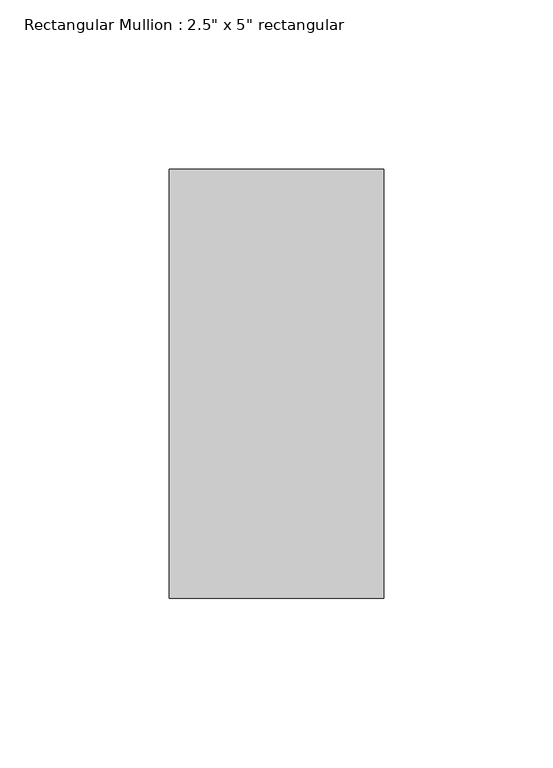
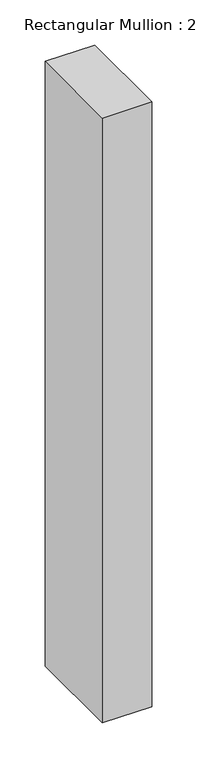
"""IFC4 building model written with IfcOpenShell, lengths in millimetres: member geometry."""

from ifc_helpers import new_model, si_unit, frame, origin, place, context, project, spatial, polyline, outline, extrude, source, transform, mapped, element, save


def member_c17f1be2(model_context):
    return source(origin(), model_context, "Body", "SweptSolid", [
        extrude(outline(polyline([(0.0, 63.5), (0.0, -63.5), (-63.5, -63.5), (-63.5, 63.5), (0.0, 63.5)])), frame((0.0, 0.0, -819.15), z_axis=(0.0, 0.0, 1.0), x_axis=(1.0, 0.0, 0.0)), (0.0, 0.0, 1.0), 819.15),
    ])


if __name__ == "__main__":
    model = new_model("IFC4")
    model_context = context("Model", 3, world=origin())
    ifc_project = project(units=[si_unit("LENGTHUNIT", "METRE", prefix="MILLI")], contexts=[model_context])
    site = spatial("IfcSite", under=ifc_project)
    building = spatial("IfcBuilding", under=site)
    placement = place(None, origin())
    member_shape = member_c17f1be2(model_context)
    element("IfcMember", 1, ObjectType="Rectangular Mullion : 2.5\" x 5\" rectangular", at=placement, inside=building, context=model_context, shape_type="MappedRepresentation", body=[
        mapped(member_shape, transform((0.0, 0.0, 0.0), x_axis=(1.0, 0.0, 0.0), y_axis=(0.0, 1.0, 0.0), z_axis=(0.0, 0.0, 1.0))),
    ])
    save(model, "model.ifc")

# Revit data of these elements
# Type "Rectangular Mullion : 2.5\" x 5\" rectangular"
#   built-in parameter 1007304 = 0.416667 (stored number, unit not read)
#   built-in parameter 1007301 = 0.104167 (stored number, unit not read)
#   built-in parameter 1007300 = 0.104167 (stored number, unit not read)
